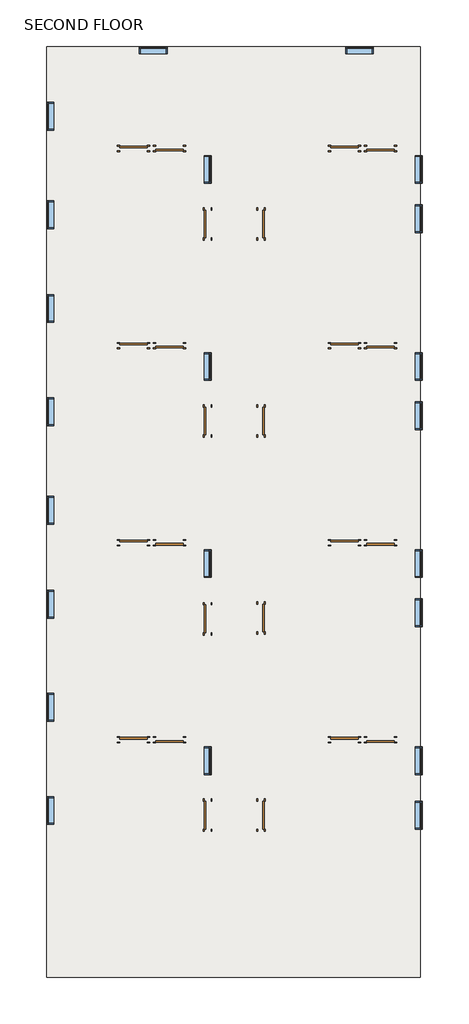
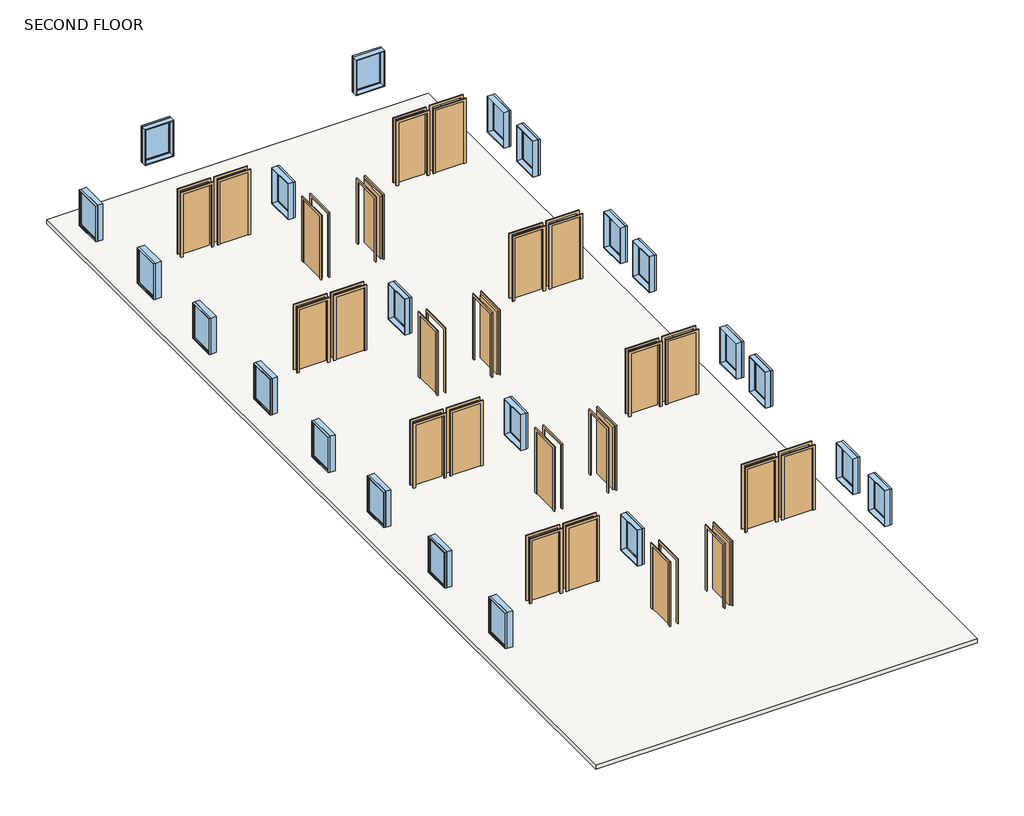
# One storey: 24 doors, 22 windows, 1 slab.
"""IFC4 building model written with IfcOpenShell, lengths in millimetres."""

from ifc_helpers import new_model, si_unit, frame, origin, place, context, project, spatial, polyline, outline, extrude, transform, mapped, element, save
from components import door_686f89d2, door_16372e1c, door_a90ba1ad, door_0ca8825f, window_c1f32544

model = new_model("IFC4")

# Units and contexts
model_context = context("Model", 3, world=origin())
ifc_project = project(units=[si_unit("LENGTHUNIT", "METRE", prefix="MILLI")], contexts=[model_context])

# Site, building, storey
site = spatial("IfcSite", under=ifc_project)
building = spatial("IfcBuilding", under=site)
storey = spatial("IfcBuildingStorey", under=building, Name="SECOND FLOOR", Elevation=6400.8)

# Doors
placement = place(None, origin())
door_shape = door_686f89d2(model_context)
element("IfcDoor", 1, ObjectType="Single-Flush : 36\" x 84\"", at=placement, inside=storey, context=model_context, shape_type="MappedRepresentation", body=[
    mapped(door_shape, transform((-9863.5902461, 11952.2710592, 6400.8), x_axis=(-1.0, 0.0, 0.0), y_axis=(0.0, -1.0, 0.0), z_axis=(0.0, 0.0, 1.0))),
])
element("IfcDoor", 2, ObjectType="Single-Flush : 36\" x 84\"", at=placement, inside=storey, context=model_context, shape_type="MappedRepresentation", body=[
    mapped(door_shape, transform((-9863.5902461, 5475.2710592, 6400.8), x_axis=(-1.0, 0.0, 0.0), y_axis=(0.0, -1.0, 0.0), z_axis=(0.0, 0.0, 1.0))),
])
element("IfcDoor", 3, ObjectType="Single-Flush : 36\" x 84\"", at=placement, inside=storey, context=model_context, shape_type="MappedRepresentation", body=[
    mapped(door_shape, transform((-9863.5902461, -1001.7289408, 6400.8), x_axis=(-1.0, 0.0, 0.0), y_axis=(0.0, -1.0, 0.0), z_axis=(0.0, 0.0, 1.0))),
])
element("IfcDoor", 4, ObjectType="Single-Flush : 36\" x 84\"", at=placement, inside=storey, context=model_context, shape_type="MappedRepresentation", body=[
    mapped(door_shape, transform((-9863.5902461, -7478.7289408, 6400.8), x_axis=(-1.0, 0.0, 0.0), y_axis=(0.0, -1.0, 0.0), z_axis=(0.0, 0.0, 1.0))),
])
element("IfcDoor", 5, ObjectType="Single-Flush : 36\" x 84\"", at=placement, inside=storey, context=model_context, shape_type="MappedRepresentation", body=[
    mapped(door_shape, transform((-2929.3902461, -7478.7289408, 6400.8), x_axis=(-1.0, 0.0, 0.0), y_axis=(0.0, -1.0, 0.0), z_axis=(0.0, 0.0, 1.0))),
])
element("IfcDoor", 6, ObjectType="Single-Flush : 36\" x 84\"", at=placement, inside=storey, context=model_context, shape_type="MappedRepresentation", body=[
    mapped(door_shape, transform((-2929.3902461, -1001.7289408, 6400.8), x_axis=(-1.0, 0.0, 0.0), y_axis=(0.0, -1.0, 0.0), z_axis=(0.0, 0.0, 1.0))),
])
element("IfcDoor", 7, ObjectType="Single-Flush : 36\" x 84\"", at=placement, inside=storey, context=model_context, shape_type="MappedRepresentation", body=[
    mapped(door_shape, transform((-2929.3902461, 5475.2710592, 6400.8), x_axis=(-1.0, 0.0, 0.0), y_axis=(0.0, -1.0, 0.0), z_axis=(0.0, 0.0, 1.0))),
])
element("IfcDoor", 8, ObjectType="Single-Flush : 36\" x 84\"", at=placement, inside=storey, context=model_context, shape_type="MappedRepresentation", body=[
    mapped(door_shape, transform((-2929.3902461, 11952.2710592, 6400.8), x_axis=(-1.0, 0.0, 0.0), y_axis=(0.0, -1.0, 0.0), z_axis=(0.0, 0.0, 1.0))),
])
door_2_shape = door_16372e1c(model_context)
element("IfcDoor", 9, ObjectType="Single-Flush : 36\" x 84\"", at=placement, inside=storey, context=model_context, shape_type="MappedRepresentation", body=[
    mapped(door_2_shape, transform((-8682.4902461, 11952.2710592, 6400.8), x_axis=(-1.0, 0.0, 0.0), y_axis=(0.0, -1.0, 0.0), z_axis=(0.0, 0.0, 1.0))),
])
element("IfcDoor", 10, ObjectType="Single-Flush : 36\" x 84\"", at=placement, inside=storey, context=model_context, shape_type="MappedRepresentation", body=[
    mapped(door_2_shape, transform((-8682.4902461, 5475.2710592, 6400.8), x_axis=(-1.0, 0.0, 0.0), y_axis=(0.0, -1.0, 0.0), z_axis=(0.0, 0.0, 1.0))),
])
element("IfcDoor", 11, ObjectType="Single-Flush : 36\" x 84\"", at=placement, inside=storey, context=model_context, shape_type="MappedRepresentation", body=[
    mapped(door_2_shape, transform((-8682.4902461, -1001.7289408, 6400.8), x_axis=(-1.0, 0.0, 0.0), y_axis=(0.0, -1.0, 0.0), z_axis=(0.0, 0.0, 1.0))),
])
element("IfcDoor", 12, ObjectType="Single-Flush : 36\" x 84\"", at=placement, inside=storey, context=model_context, shape_type="MappedRepresentation", body=[
    mapped(door_2_shape, transform((-8682.4902461, -7478.7289408, 6400.8), x_axis=(-1.0, 0.0, 0.0), y_axis=(0.0, -1.0, 0.0), z_axis=(0.0, 0.0, 1.0))),
])
element("IfcDoor", 13, ObjectType="Single-Flush : 36\" x 84\"", at=placement, inside=storey, context=model_context, shape_type="MappedRepresentation", body=[
    mapped(door_2_shape, transform((-1748.2902461, -7478.7289408, 6400.8), x_axis=(-1.0, 0.0, 0.0), y_axis=(0.0, -1.0, 0.0), z_axis=(0.0, 0.0, 1.0))),
])
element("IfcDoor", 14, ObjectType="Single-Flush : 36\" x 84\"", at=placement, inside=storey, context=model_context, shape_type="MappedRepresentation", body=[
    mapped(door_2_shape, transform((-1748.2902461, -1001.7289408, 6400.8), x_axis=(-1.0, 0.0, 0.0), y_axis=(0.0, -1.0, 0.0), z_axis=(0.0, 0.0, 1.0))),
])
element("IfcDoor", 15, ObjectType="Single-Flush : 36\" x 84\"", at=placement, inside=storey, context=model_context, shape_type="MappedRepresentation", body=[
    mapped(door_2_shape, transform((-1748.2902461, 5475.2710592, 6400.8), x_axis=(-1.0, 0.0, 0.0), y_axis=(0.0, -1.0, 0.0), z_axis=(0.0, 0.0, 1.0))),
])
element("IfcDoor", 16, ObjectType="Single-Flush : 36\" x 84\"", at=placement, inside=storey, context=model_context, shape_type="MappedRepresentation", body=[
    mapped(door_2_shape, transform((-1748.2902461, 11952.2710592, 6400.8), x_axis=(-1.0, 0.0, 0.0), y_axis=(0.0, -1.0, 0.0), z_axis=(0.0, 0.0, 1.0))),
])
door_3_shape = door_a90ba1ad(model_context)
element("IfcDoor", 17, ObjectType="Single-Flush : 36\" x 84\"", at=placement, inside=storey, context=model_context, shape_type="MappedRepresentation", body=[
    mapped(door_3_shape, transform((-7425.1902461, 9475.7710592, 6400.8), x_axis=(0.0, -1.0, 0.0), y_axis=(1.0, 0.0, 0.0), z_axis=(0.0, 0.0, 1.0))),
])
element("IfcDoor", 18, ObjectType="Single-Flush : 36\" x 84\"", at=placement, inside=storey, context=model_context, shape_type="MappedRepresentation", body=[
    mapped(door_3_shape, transform((-7425.1902461, 2998.7710592, 6400.8), x_axis=(0.0, -1.0, 0.0), y_axis=(1.0, 0.0, 0.0), z_axis=(0.0, 0.0, 1.0))),
])
element("IfcDoor", 19, ObjectType="Single-Flush : 36\" x 84\"", at=placement, inside=storey, context=model_context, shape_type="MappedRepresentation", body=[
    mapped(door_3_shape, transform((-7425.1902461, -9955.2289408, 6400.8), x_axis=(0.0, -1.0, 0.0), y_axis=(1.0, 0.0, 0.0), z_axis=(0.0, 0.0, 1.0))),
])
element("IfcDoor", 20, ObjectType="Single-Flush : 36\" x 84\"", at=placement, inside=storey, context=model_context, shape_type="MappedRepresentation", body=[
    mapped(door_3_shape, transform((-7425.1902461, -3503.6289408, 6400.8), x_axis=(0.0, -1.0, 0.0), y_axis=(1.0, 0.0, 0.0), z_axis=(0.0, 0.0, 1.0))),
])
door_4_shape = door_0ca8825f(model_context)
element("IfcDoor", 21, ObjectType="Single-Flush : 36\" x 84\"", at=placement, inside=storey, context=model_context, shape_type="MappedRepresentation", body=[
    mapped(door_4_shape, transform((-5672.5902461, 9475.7710592, 6400.8), x_axis=(0.0, -1.0, 0.0), y_axis=(1.0, 0.0, 0.0), z_axis=(0.0, 0.0, 1.0))),
])
element("IfcDoor", 22, ObjectType="Single-Flush : 36\" x 84\"", at=placement, inside=storey, context=model_context, shape_type="MappedRepresentation", body=[
    mapped(door_4_shape, transform((-5672.5902461, 2998.7710592, 6400.8), x_axis=(0.0, -1.0, 0.0), y_axis=(1.0, 0.0, 0.0), z_axis=(0.0, 0.0, 1.0))),
])
element("IfcDoor", 23, ObjectType="Single-Flush : 36\" x 84\"", at=placement, inside=storey, context=model_context, shape_type="MappedRepresentation", body=[
    mapped(door_4_shape, transform((-5672.5902461, -9955.2289408, 6400.8), x_axis=(0.0, -1.0, 0.0), y_axis=(1.0, 0.0, 0.0), z_axis=(0.0, 0.0, 1.0))),
])
element("IfcDoor", 24, ObjectType="Single-Flush : 36\" x 84\"", at=placement, inside=storey, context=model_context, shape_type="MappedRepresentation", body=[
    mapped(door_4_shape, transform((-5672.5902461, -3478.2289408, 6400.8), x_axis=(0.0, -1.0, 0.0), y_axis=(1.0, 0.0, 0.0), z_axis=(0.0, 0.0, 1.0))),
])

# Slab
element("IfcSlab", 25, ObjectType="Generic - 12\"", at=placement, inside=storey, context=model_context, shape_type="SweptSolid", body=[
    extrude(outline(polyline([(-440.1902461, 15305.0710592), (-440.1902461, -15289.2289408), (-12721.0902461, -15289.2289408), (-12721.0902461, 15305.0710592), (-440.1902461, 15305.0710592)])), frame((0.0, 0.0, 6273.8), z_axis=(0.0, 0.0, 1.0), x_axis=(1.0, 0.0, 0.0)), (0.0, 0.0, 1.0), 127.0),
])

# Windows
window_shape = window_c1f32544(model_context)
element("IfcWindow", 26, ObjectType="Fixed : 36\" x 48\"", at=placement, inside=storey, context=model_context, shape_type="MappedRepresentation", body=[
    mapped(window_shape, transform((-9177.7902461, 15190.7710592, 6400.8), x_axis=(1.0, 0.0, 0.0), y_axis=(0.0, 1.0, 0.0), z_axis=(0.0, 0.0, 1.0))),
])
element("IfcWindow", 27, ObjectType="Fixed : 36\" x 48\"", at=placement, inside=storey, context=model_context, shape_type="MappedRepresentation", body=[
    mapped(window_shape, transform((-12606.7902461, 13057.1710592, 6400.8), x_axis=(0.0, 1.0, 0.0), y_axis=(-1.0, 0.0, 0.0), z_axis=(0.0, 0.0, 1.0))),
])
element("IfcWindow", 28, ObjectType="Fixed : 36\" x 48\"", at=placement, inside=storey, context=model_context, shape_type="MappedRepresentation", body=[
    mapped(window_shape, transform((-12606.7902461, 9818.6710592, 6400.8), x_axis=(0.0, 1.0, 0.0), y_axis=(-1.0, 0.0, 0.0), z_axis=(0.0, 0.0, 1.0))),
])
element("IfcWindow", 29, ObjectType="Fixed : 36\" x 48\"", at=placement, inside=storey, context=model_context, shape_type="MappedRepresentation", body=[
    mapped(window_shape, transform((-12606.7902461, 6732.5710592, 6400.8), x_axis=(0.0, 1.0, 0.0), y_axis=(-1.0, 0.0, 0.0), z_axis=(0.0, 0.0, 1.0))),
])
element("IfcWindow", 30, ObjectType="Fixed : 36\" x 48\"", at=placement, inside=storey, context=model_context, shape_type="MappedRepresentation", body=[
    mapped(window_shape, transform((-12606.7902461, 3341.6710592, 6400.8), x_axis=(0.0, 1.0, 0.0), y_axis=(-1.0, 0.0, 0.0), z_axis=(0.0, 0.0, 1.0))),
])
element("IfcWindow", 31, ObjectType="Fixed : 36\" x 48\"", at=placement, inside=storey, context=model_context, shape_type="MappedRepresentation", body=[
    mapped(window_shape, transform((-12606.7902461, 103.1710592, 6400.8), x_axis=(0.0, 1.0, 0.0), y_axis=(-1.0, 0.0, 0.0), z_axis=(0.0, 0.0, 1.0))),
])
element("IfcWindow", 32, ObjectType="Fixed : 36\" x 48\"", at=placement, inside=storey, context=model_context, shape_type="MappedRepresentation", body=[
    mapped(window_shape, transform((-12606.7902461, -2982.9289408, 6400.8), x_axis=(0.0, 1.0, 0.0), y_axis=(-1.0, 0.0, 0.0), z_axis=(0.0, 0.0, 1.0))),
])
element("IfcWindow", 33, ObjectType="Fixed : 36\" x 48\"", at=placement, inside=storey, context=model_context, shape_type="MappedRepresentation", body=[
    mapped(window_shape, transform((-12606.7902461, -6373.8289408, 6400.8), x_axis=(0.0, 1.0, 0.0), y_axis=(-1.0, 0.0, 0.0), z_axis=(0.0, 0.0, 1.0))),
])
element("IfcWindow", 34, ObjectType="Fixed : 36\" x 48\"", at=placement, inside=storey, context=model_context, shape_type="MappedRepresentation", body=[
    mapped(window_shape, transform((-12606.7902461, -9764.7289408, 6400.8), x_axis=(0.0, 1.0, 0.0), y_axis=(-1.0, 0.0, 0.0), z_axis=(0.0, 0.0, 1.0))),
])
element("IfcWindow", 35, ObjectType="Fixed : 36\" x 48\"", at=placement, inside=storey, context=model_context, shape_type="MappedRepresentation", body=[
    mapped(window_shape, transform((-7425.1902461, -8202.6289408, 6400.8), x_axis=(0.0, -1.0, 0.0), y_axis=(1.0, 0.0, 0.0), z_axis=(0.0, 0.0, 1.0))),
])
element("IfcWindow", 36, ObjectType="Fixed : 36\" x 48\"", at=placement, inside=storey, context=model_context, shape_type="MappedRepresentation", body=[
    mapped(window_shape, transform((-7425.1902461, -1725.6289408, 6400.8), x_axis=(0.0, -1.0, 0.0), y_axis=(1.0, 0.0, 0.0), z_axis=(0.0, 0.0, 1.0))),
])
element("IfcWindow", 37, ObjectType="Fixed : 36\" x 48\"", at=placement, inside=storey, context=model_context, shape_type="MappedRepresentation", body=[
    mapped(window_shape, transform((-7425.1902461, 4751.3710592, 6400.8), x_axis=(0.0, -1.0, 0.0), y_axis=(1.0, 0.0, 0.0), z_axis=(0.0, 0.0, 1.0))),
])
element("IfcWindow", 38, ObjectType="Fixed : 36\" x 48\"", at=placement, inside=storey, context=model_context, shape_type="MappedRepresentation", body=[
    mapped(window_shape, transform((-7425.1902461, 11228.3710592, 6400.8), x_axis=(0.0, -1.0, 0.0), y_axis=(1.0, 0.0, 0.0), z_axis=(0.0, 0.0, 1.0))),
])
element("IfcWindow", 39, ObjectType="Fixed : 36\" x 48\"", at=placement, inside=storey, context=model_context, shape_type="MappedRepresentation", body=[
    mapped(window_shape, transform((-490.9902461, 11228.3710592, 6400.8), x_axis=(0.0, -1.0, 0.0), y_axis=(1.0, 0.0, 0.0), z_axis=(0.0, 0.0, 1.0))),
])
element("IfcWindow", 40, ObjectType="Fixed : 36\" x 48\"", at=placement, inside=storey, context=model_context, shape_type="MappedRepresentation", body=[
    mapped(window_shape, transform((-490.9902461, 9609.1210592, 6400.8), x_axis=(0.0, -1.0, 0.0), y_axis=(1.0, 0.0, 0.0), z_axis=(0.0, 0.0, 1.0))),
])
element("IfcWindow", 41, ObjectType="Fixed : 36\" x 48\"", at=placement, inside=storey, context=model_context, shape_type="MappedRepresentation", body=[
    mapped(window_shape, transform((-490.9902461, 4751.3710592, 6400.8), x_axis=(0.0, -1.0, 0.0), y_axis=(1.0, 0.0, 0.0), z_axis=(0.0, 0.0, 1.0))),
])
element("IfcWindow", 42, ObjectType="Fixed : 36\" x 48\"", at=placement, inside=storey, context=model_context, shape_type="MappedRepresentation", body=[
    mapped(window_shape, transform((-490.9902461, 3132.1210592, 6400.8), x_axis=(0.0, -1.0, 0.0), y_axis=(1.0, 0.0, 0.0), z_axis=(0.0, 0.0, 1.0))),
])
element("IfcWindow", 43, ObjectType="Fixed : 36\" x 48\"", at=placement, inside=storey, context=model_context, shape_type="MappedRepresentation", body=[
    mapped(window_shape, transform((-490.9902461, -1725.6289408, 6400.8), x_axis=(0.0, -1.0, 0.0), y_axis=(1.0, 0.0, 0.0), z_axis=(0.0, 0.0, 1.0))),
])
element("IfcWindow", 44, ObjectType="Fixed : 36\" x 48\"", at=placement, inside=storey, context=model_context, shape_type="MappedRepresentation", body=[
    mapped(window_shape, transform((-490.9902461, -3344.8789408, 6400.8), x_axis=(0.0, -1.0, 0.0), y_axis=(1.0, 0.0, 0.0), z_axis=(0.0, 0.0, 1.0))),
])
element("IfcWindow", 45, ObjectType="Fixed : 36\" x 48\"", at=placement, inside=storey, context=model_context, shape_type="MappedRepresentation", body=[
    mapped(window_shape, transform((-490.9902461, -8202.6289408, 6400.8), x_axis=(0.0, -1.0, 0.0), y_axis=(1.0, 0.0, 0.0), z_axis=(0.0, 0.0, 1.0))),
])
element("IfcWindow", 46, ObjectType="Fixed : 36\" x 48\"", at=placement, inside=storey, context=model_context, shape_type="MappedRepresentation", body=[
    mapped(window_shape, transform((-490.9902461, -9993.3289408, 6400.8), x_axis=(0.0, -1.0, 0.0), y_axis=(1.0, 0.0, 0.0), z_axis=(0.0, 0.0, 1.0))),
])
element("IfcWindow", 47, ObjectType="Fixed : 36\" x 48\"", at=placement, inside=storey, context=model_context, shape_type="MappedRepresentation", body=[
    mapped(window_shape, transform((-2395.9902461, 15190.7710592, 6400.8), x_axis=(1.0, 0.0, 0.0), y_axis=(0.0, 1.0, 0.0), z_axis=(0.0, 0.0, 1.0))),
])

save(model, "model.ifc")

# Revit data of these elements
# Type "Single-Flush : 36\" x 84\""
#   Type Mark = "1"
#   Construction Type Id = "MDOOR"
#   Assembly Code = "C1020"
#   Analytic Construction = "Metal"
#   Thickness = 0' - 2"
#   Heat Transfer Coefficient (U) = 0.651978 BTU/(h·ft²·°F)
#   Height = 7' - 0"
#   Trim Projection Ext = 0' - 1"
#   Trim Projection Int = 0' - 1"
#   Trim Width = 0' - 3"
#   Width = 3' - 0"
#   Define Thermal Properties by = 1
#   Door Material = Door - Panel
#   Frame Material = Door - Frame
#   Visual Light Transmittance = 0
#   Solar Heat Gain Coefficient = 0
#   Function = (empty or 0)
#   Wall Closure = (empty or 0)
# Type "Generic - 12\""
#   Assembly Code = "B1010"
#   Function = 0
#   Layers, outside or top first: 0' - 5" no material (function 1)
# Type "Fixed : 36\" x 48\""
#   Type Mark = "1"
#   Construction Type Id = "GSP4R"
#   Assembly Code = "B2020100"
#   Analytic Construction = "1/8 in Pilkington single glazing"
#   Visual Light Transmittance = 0.9
#   Solar Heat Gain Coefficient = 0.78
#   Heat Transfer Coefficient (U) = 0.6496 BTU/(h·ft²·°F)
#   Height = 4' - 0"
#   Default Sill Height = 3' - 0"
#   Width = 3' - 0"
#   Window Inset = 0' - 0 3/4"
#   Define Thermal Properties by = 1
#   Glass Pane Material = Glass
#   Sash Material = Sash
#   Wall Closure = (empty or 0)
# Elements 1, 2, 3, 4, 5, 6, 7, 8, 9, 10, 11, 12, 13, 14, 15, 16, 17, 18, 19, 20, 21, 22, 23, 24 (IfcDoor, "Single-Flush : 36\" x 84\"")
#   Phase Created = New Construction
#   Materials on its faces: "Door - Frame", "Door - Panel"
# Element 25 (IfcSlab, "Generic - 12\"")
#   Height Offset From Level = 0' - 0"
#   Phase Created = New Construction
#   Materials on its faces: "Default Floor"
# Element 26 (IfcWindow, "Fixed : 36\" x 48\"")
#   Mark = "49"
#   Phase Created = New Construction
#   Materials on its faces: "Sash", "Glass"
# Element 27 (IfcWindow, "Fixed : 36\" x 48\"")
#   Mark = "50"
#   Phase Created = New Construction
#   Materials on its faces: "Sash", "Glass"
# Element 28 (IfcWindow, "Fixed : 36\" x 48\"")
#   Mark = "51"
#   Phase Created = New Construction
#   Materials on its faces: "Sash", "Glass"
# Element 29 (IfcWindow, "Fixed : 36\" x 48\"")
#   Mark = "52"
#   Phase Created = New Construction
#   Materials on its faces: "Sash", "Glass"
# Element 30 (IfcWindow, "Fixed : 36\" x 48\"")
#   Mark = "53"
#   Phase Created = New Construction
#   Materials on its faces: "Sash", "Glass"
# Element 31 (IfcWindow, "Fixed : 36\" x 48\"")
#   Mark = "54"
#   Phase Created = New Construction
#   Materials on its faces: "Sash", "Glass"
# Element 32 (IfcWindow, "Fixed : 36\" x 48\"")
#   Mark = "55"
#   Phase Created = New Construction
#   Materials on its faces: "Sash", "Glass"
# Element 33 (IfcWindow, "Fixed : 36\" x 48\"")
#   Mark = "56"
#   Phase Created = New Construction
#   Materials on its faces: "Sash", "Glass"
# Element 34 (IfcWindow, "Fixed : 36\" x 48\"")
#   Mark = "57"
#   Phase Created = New Construction
#   Materials on its faces: "Sash", "Glass"
# Element 35 (IfcWindow, "Fixed : 36\" x 48\"")
#   Mark = "58"
#   Phase Created = New Construction
#   Materials on its faces: "Sash", "Glass"
# Element 36 (IfcWindow, "Fixed : 36\" x 48\"")
#   Mark = "59"
#   Phase Created = New Construction
#   Materials on its faces: "Sash", "Glass"
# Element 37 (IfcWindow, "Fixed : 36\" x 48\"")
#   Mark = "60"
#   Phase Created = New Construction
#   Materials on its faces: "Sash", "Glass"
# Element 38 (IfcWindow, "Fixed : 36\" x 48\"")
#   Mark = "61"
#   Phase Created = New Construction
#   Materials on its faces: "Sash", "Glass"
# Element 39 (IfcWindow, "Fixed : 36\" x 48\"")
#   Mark = "62"
#   Phase Created = New Construction
#   Materials on its faces: "Sash", "Glass"
# Element 40 (IfcWindow, "Fixed : 36\" x 48\"")
#   Mark = "63"
#   Phase Created = New Construction
#   Materials on its faces: "Sash", "Glass"
# Element 41 (IfcWindow, "Fixed : 36\" x 48\"")
#   Mark = "64"
#   Phase Created = New Construction
#   Materials on its faces: "Sash", "Glass"
# Element 42 (IfcWindow, "Fixed : 36\" x 48\"")
#   Mark = "65"
#   Phase Created = New Construction
#   Materials on its faces: "Sash", "Glass"
# Element 43 (IfcWindow, "Fixed : 36\" x 48\"")
#   Mark = "66"
#   Phase Created = New Construction
#   Materials on its faces: "Sash", "Glass"
# Element 44 (IfcWindow, "Fixed : 36\" x 48\"")
#   Mark = "67"
#   Phase Created = New Construction
#   Materials on its faces: "Sash", "Glass"
# Element 45 (IfcWindow, "Fixed : 36\" x 48\"")
#   Mark = "68"
#   Phase Created = New Construction
#   Materials on its faces: "Sash", "Glass"
# Element 46 (IfcWindow, "Fixed : 36\" x 48\"")
#   Mark = "69"
#   Phase Created = New Construction
#   Materials on its faces: "Sash", "Glass"
# Element 47 (IfcWindow, "Fixed : 36\" x 48\"")
#   Mark = "70"
#   Phase Created = New Construction
#   Materials on its faces: "Sash", "Glass"
# Materials
#   "Door - Panel": class "Wood", colour RGB 210 159 95, transparency 0
#   "Door - Frame": colour RGB 118 70 51, transparency 0
#   "Glass": class "Glass", colour RGB 0 128 192, transparency 0.75, Description = "Soda Lime Glass", Cost = 0
#   "Sash": class "Wood", colour RGB 224 178 126, transparency 0
#   "Default Floor": colour RGB 128 128 128, transparency 0
